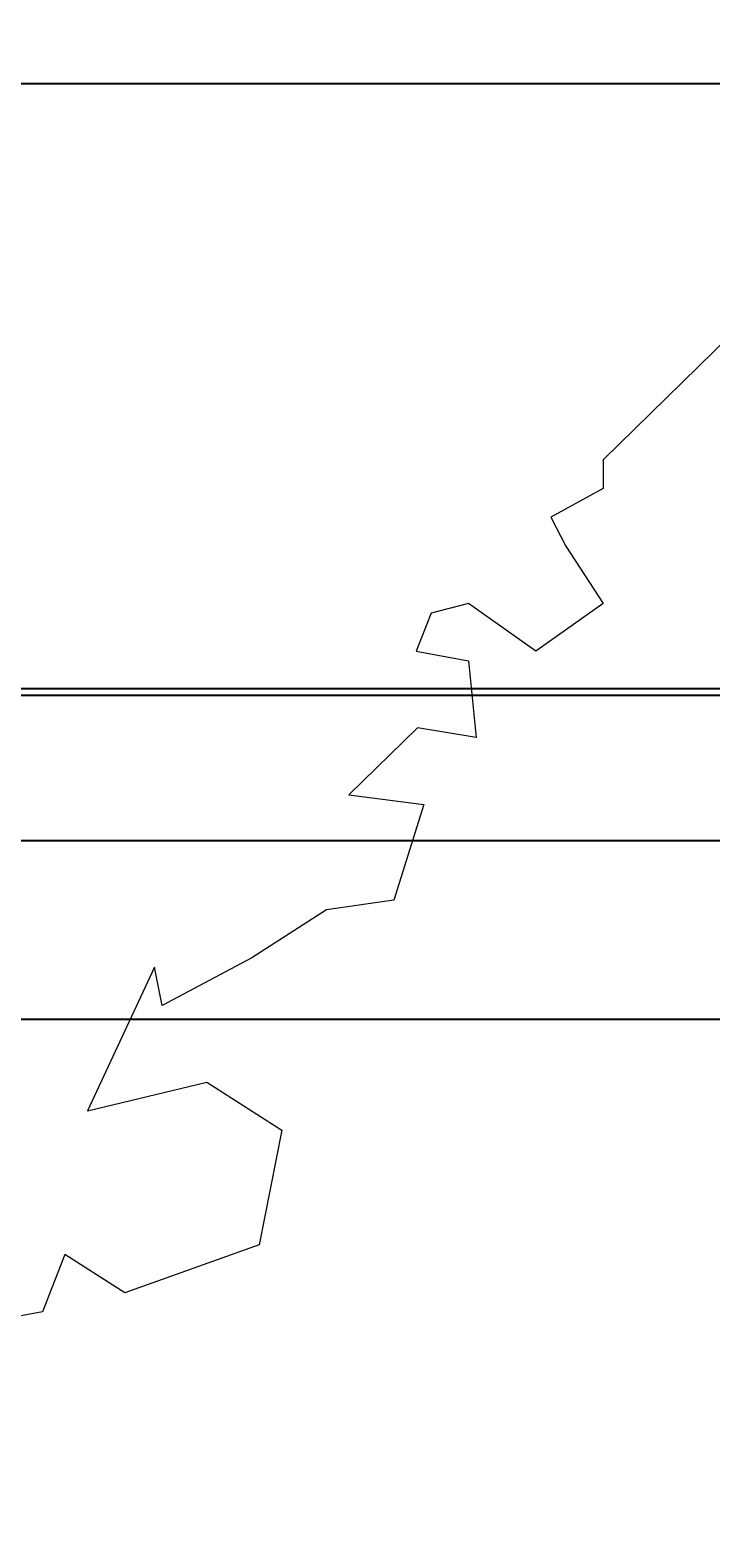
# Model space of a CAD drawing. Units: inches. Extents: x -26 to 776, y -22 to 650.
# Tile 50 of 62: x 586 to 642, y 102 to 226. Entities that reach past the tile are written whole.
import ezdxf

# ---------------------------------------------------------------- set-up
doc = ezdxf.new("R2010")
doc.units = ezdxf.units.IN
doc.header["$MEASUREMENT"] = 0
doc.layers.add('A-ANNO-DIMS', color=2, linetype='Continuous', lineweight=18)
doc.layers.add('L-PLNT-TREE', color=94, linetype='Continuous', lineweight=18)
doc.styles.get("Standard").update_dxf_attribs({"font": 'arial.ttf'})
doc.dimstyles.get("Standard").update_dxf_attribs({"dimtxt": 0.5625, "dimasz": 0.18, "dimexe": 0.18, "dimexo": 0.0625, "dimgap": 0.09, "dimtad": 0, "dimtih": 1, "dimtoh": 1, "dimdec": 4, "dimzin": 0, "dimdsep": 46, "dimlunit": 4, "dimtxsty": 'Standard', "dimcen": 0.09, "dimadec": 0, "dimazin": 0, "dimtfac": 1, "dimtdec": 4, "dimtofl": 0, "dimtmove": 0, "dimatfit": 3, "dimfxl": 1, "dimtolj": 1, "dimtzin": 0, "dimarcsym": 0})

# ---------------------------------------------------------------- blocks, each defined once
blk = doc.blocks.new('Tree - type 3 evergreen elevation')
blk.add_lwpolyline([(0.4313, 130.5029), (-6.9015, 123.3141), (-6.9015, 121.6552), (-9.9208, 119.9963), (-9.0581, 118.3373), (-6.9015, 115.0195), (-10.7835, 112.2546), (-14.6656, 115.0195), (-16.8222, 114.4665), (-17.6849, 112.2546), (-14.6656, 111.7016), (-14.2342, 107.2778), (-17.6065, 107.8307), (-21.5669, 103.9599), (-17.2536, 103.4069), (-18.9789, 97.8771), (-22.8609, 97.3241), (-27.1743, 94.5593), (-32.3504, 91.7944), (-32.7817, 94.0063), (-36.6638, 85.7116), (-29.7624, 87.3705), (-25.449, 84.6056), (-26.743, 77.9699), (-34.507, 75.205), (-37.9578, 77.4169), (-39.2518, 74.099), (-42.2711, 73.5461)])
blk = doc.blocks.new('*D20')
at = {"layer": 'A-ANNO-DIMS', "color": 0, "lineweight": -2, "transparency": 16777216}
for p, q in [((425.81, 455.47), (775.34, 455.47)), ((775.16, 455.29), (775.16, 235.85)), ((775.16, 15.66), (775.16, 235.1)), ((425.81, 15.48), (775.34, 15.48))]:
    blk.add_line(p, q, dxfattribs=at)
at = {"layer": 'A-ANNO-DIMS', "color": 0, "transparency": 16777216}
for points in [[(775.13, 455.29), (775.19, 455.29), (775.16, 455.47)], [(775.13, 15.66), (775.19, 15.66), (775.16, 15.48)]]:
    blk.add_solid(points, dxfattribs=at)
at = {"layer": 'Defpoints', "color": 0, "transparency": 16777216}
for p in [(425.74, 455.47), (775.16, 455.47), (425.74, 15.48)]:
    blk.add_point(p, dxfattribs=at)
at = {"layer": 'A-ANNO-DIMS', "color": 0, "transparency": 16777216, "insert": (775.16, 235.48), "char_height": 0.562, "attachment_point": 5}
blk.add_mtext('\\A1;440', dxfattribs=at)
blk = doc.blocks.new('*D26')
at = {"layer": 'A-ANNO-DIMS', "color": 0, "lineweight": -2, "transparency": 16777216}
for p, q in [((91.71, 171.97), (775.34, 171.97)), ((775.16, 171.79), (775.16, 166.11)), ((775.16, 159.66), (775.16, 165.35)), ((82.2, 159.48), (775.34, 159.48))]:
    blk.add_line(p, q, dxfattribs=at)
at = {"layer": 'A-ANNO-DIMS', "color": 0, "transparency": 16777216}
for points in [[(775.13, 171.79), (775.19, 171.79), (775.16, 171.97)], [(775.13, 159.66), (775.19, 159.66), (775.16, 159.48)]]:
    blk.add_solid(points, dxfattribs=at)
at = {"layer": 'Defpoints', "color": 0, "transparency": 16777216}
for p in [(91.64, 171.97), (775.16, 171.97), (82.13, 159.48)]:
    blk.add_point(p, dxfattribs=at)
at = {"layer": 'A-ANNO-DIMS', "color": 0, "transparency": 16777216, "insert": (775.16, 165.73), "char_height": 0.562, "attachment_point": 5}
blk.add_mtext('\\A1;12.49', dxfattribs=at)
blk = doc.blocks.new('*D28')
at = {"layer": 'A-ANNO-DIMS', "color": 0, "lineweight": -2, "transparency": 16777216}
for p, q in [((285.08, 314.12), (775.34, 314.12)), ((775.16, 313.94), (775.16, 243.14)), ((775.16, 171.6), (775.16, 242.4)), ((285.08, 171.42), (775.34, 171.42))]:
    blk.add_line(p, q, dxfattribs=at)
at = {"layer": 'A-ANNO-DIMS', "color": 0, "transparency": 16777216}
for points in [[(775.13, 313.94), (775.19, 313.94), (775.16, 314.12)], [(775.13, 171.6), (775.19, 171.6), (775.16, 171.42)]]:
    blk.add_solid(points, dxfattribs=at)
at = {"layer": 'Defpoints', "color": 0, "transparency": 16777216}
for p in [(285.02, 314.12), (775.16, 314.12), (285.02, 171.42)]:
    blk.add_point(p, dxfattribs=at)
at = {"layer": 'A-ANNO-DIMS', "color": 0, "transparency": 16777216, "insert": (775.16, 242.77), "char_height": 0.562, "attachment_point": 5}
blk.add_mtext('\\A1;142.7', dxfattribs=at)
blk = doc.blocks.new('*D30')
at = {"layer": 'A-ANNO-DIMS', "color": 0, "lineweight": -2, "transparency": 16777216}
for p, q in [((280.68, 144.84), (775.34, 144.84)), ((775.16, 144.66), (775.16, 86.01)), ((775.16, 26.6), (775.16, 85.25)), ((280.68, 26.42), (775.34, 26.42))]:
    blk.add_line(p, q, dxfattribs=at)
at = {"layer": 'A-ANNO-DIMS', "color": 0, "transparency": 16777216}
for points in [[(775.13, 144.66), (775.19, 144.66), (775.16, 144.84)], [(775.13, 26.6), (775.19, 26.6), (775.16, 26.42)]]:
    blk.add_solid(points, dxfattribs=at)
at = {"layer": 'Defpoints', "color": 0, "transparency": 16777216}
for p in [(280.62, 144.84), (775.16, 144.84), (280.62, 26.42)]:
    blk.add_point(p, dxfattribs=at)
at = {"layer": 'A-ANNO-DIMS', "color": 0, "transparency": 16777216, "insert": (775.16, 85.63), "char_height": 0.562, "attachment_point": 5}
blk.add_mtext('\\A1;118.41', dxfattribs=at)
blk = doc.blocks.new('*D41')
at = {"layer": 'A-ANNO-DIMS', "color": 0, "lineweight": -2, "transparency": 16777216}
for p, q in [((11.17, 221.64), (775.34, 221.64)), ((775.16, 221.46), (775.16, 190.94)), ((775.16, 159.66), (775.16, 190.18)), ((11.17, 159.48), (775.34, 159.48))]:
    blk.add_line(p, q, dxfattribs=at)
at = {"layer": 'A-ANNO-DIMS', "color": 0, "transparency": 16777216}
for points in [[(775.13, 221.46), (775.19, 221.46), (775.16, 221.64)], [(775.13, 159.66), (775.19, 159.66), (775.16, 159.48)]]:
    blk.add_solid(points, dxfattribs=at)
at = {"layer": 'Defpoints', "color": 0, "transparency": 16777216}
for p in [(11.11, 221.64), (775.16, 221.64), (11.11, 159.48)]:
    blk.add_point(p, dxfattribs=at)
at = {"layer": 'A-ANNO-DIMS', "color": 0, "transparency": 16777216, "insert": (775.16, 190.56), "char_height": 0.562, "attachment_point": 5}
blk.add_mtext('\\A1;62.16', dxfattribs=at)
blk = doc.blocks.new('*D42')
at = {"layer": 'A-ANNO-DIMS', "color": 0, "lineweight": -2, "transparency": 16777216}
for p, q in [((285.08, 171.42), (775.34, 171.42)), ((775.16, 171.24), (775.16, 165.83)), ((775.16, 159.66), (775.16, 165.07)), ((289.3, 159.48), (775.34, 159.48))]:
    blk.add_line(p, q, dxfattribs=at)
at = {"layer": 'A-ANNO-DIMS', "color": 0, "transparency": 16777216}
for points in [[(775.13, 171.24), (775.19, 171.24), (775.16, 171.42)], [(775.13, 159.66), (775.19, 159.66), (775.16, 159.48)]]:
    blk.add_solid(points, dxfattribs=at)
at = {"layer": 'Defpoints', "color": 0, "transparency": 16777216}
for p in [(285.02, 171.42), (775.16, 171.42), (289.24, 159.48)]:
    blk.add_point(p, dxfattribs=at)
at = {"layer": 'A-ANNO-DIMS', "color": 0, "transparency": 16777216, "insert": (775.16, 165.45), "char_height": 0.562, "attachment_point": 5}
blk.add_mtext('\\A1;11.935', dxfattribs=at)
blk = doc.blocks.new('*D45')
at = {"layer": 'A-ANNO-DIMS', "color": 0, "lineweight": -2, "transparency": 16777216}
for p, q in [((507.74, 408.64), (775.34, 408.64)), ((775.16, 408.46), (775.16, 212.44)), ((775.16, 15.66), (775.16, 211.68)), ((586, 15.48), (775.34, 15.48))]:
    blk.add_line(p, q, dxfattribs=at)
at = {"layer": 'A-ANNO-DIMS', "color": 0, "transparency": 16777216}
for points in [[(775.13, 408.46), (775.19, 408.46), (775.16, 408.64)], [(775.13, 15.66), (775.19, 15.66), (775.16, 15.48)]]:
    blk.add_solid(points, dxfattribs=at)
at = {"layer": 'Defpoints', "color": 0, "transparency": 16777216}
for p in [(507.68, 408.64), (775.16, 408.64), (585.94, 15.48)]:
    blk.add_point(p, dxfattribs=at)
at = {"layer": 'A-ANNO-DIMS', "color": 0, "transparency": 16777216, "insert": (775.16, 212.06), "char_height": 0.562, "attachment_point": 5}
blk.add_mtext('\\A1;393.16', dxfattribs=at)
blk = doc.blocks.new('*D48')
at = {"layer": 'A-ANNO-DIMS', "color": 0, "lineweight": -2, "transparency": 16777216}
for p, q in [((545.03, 67.41), (545.03, 649.86)), ((738.75, 50.91), (738.75, 649.86)), ((545.21, 649.68), (640.88, 649.68)), ((738.57, 649.68), (642.9, 649.68))]:
    blk.add_line(p, q, dxfattribs=at)
at = {"layer": 'A-ANNO-DIMS', "color": 0, "transparency": 16777216}
for points in [[(545.21, 649.71), (545.21, 649.65), (545.03, 649.68)], [(738.57, 649.71), (738.57, 649.65), (738.75, 649.68)]]:
    blk.add_solid(points, dxfattribs=at)
at = {"layer": 'Defpoints', "color": 0, "transparency": 16777216}
for p in [(738.75, 649.68), (545.03, 67.35), (738.75, 50.85)]:
    blk.add_point(p, dxfattribs=at)
at = {"layer": 'A-ANNO-DIMS', "color": 0, "transparency": 16777216, "insert": (641.89, 649.68), "char_height": 0.562, "attachment_point": 5}
blk.add_mtext('\\A1;193.7', dxfattribs=at)

msp = doc.modelspace()

# ---------------------------------------------------------------- block references
at = {"layer": 'L-PLNT-TREE', "xscale": 1.421226385586178, "yscale": 1.421226385586178, "zscale": 1.421226385586178}
msp.add_blockref('Tree - type 3 evergreen elevation', (642.5048, 15.4824), dxfattribs=at)

# ---------------------------------------------------------------- dimensions: what is measured, and where the dimension line sits
at = {"layer": 'A-ANNO-DIMS'}
dim = msp.add_linear_dim(base=(738.7503, 649.6763), p1=(545.0331, 67.3523), p2=(738.7503, 50.8482), dimstyle='Standard', override={"dimdec": 1, "dimlfac": 1, "dimrnd": 0, "dimzin": 0, "dimdsep": 46, "dimlunit": 2}, dxfattribs=at)
dim.commit()
dim.dimension.update_dxf_attribs({"geometry": '*D48', "text_midpoint": (641.8917, 649.6763)})
for base, p1, p2, override, picture, middle in [((775.1553, 455.4717), (425.7434, 15.4824), (425.7434, 455.4717), {"dimdec": 0, "dimlfac": 1, "dimrnd": 0, "dimzin": 0, "dimdsep": 46, "dimlunit": 2}, '*D20', (775.1553, 235.477)), ((775.1553, 408.6389), (585.9354, 15.4824), (507.6759, 408.6389), {"dimdec": 2, "dimlfac": 1, "dimrnd": 0, "dimzin": 0, "dimdsep": 46, "dimlunit": 2}, '*D45', (775.1553, 212.0606)), ((775.1553, 314.119), (285.0179, 171.4173), (285.0179, 314.119), {"dimdec": 1, "dimlfac": 1, "dimrnd": 0, "dimzin": 0, "dimdsep": 46, "dimlunit": 2}, '*D28', (775.1553, 242.7682)), ((775.1553, 221.6413), (11.1074, 159.4824), (11.1074, 221.6413), {"dimdec": 2, "dimlfac": 1, "dimrnd": 0, "dimzin": 0, "dimdsep": 46, "dimlunit": 2}, '*D41', (775.1553, 190.5618)), ((775.1553, 171.9734), (82.134, 159.4824), (91.6448, 171.9734), {"dimdec": 2, "dimlfac": 1, "dimrnd": 0, "dimzin": 0, "dimdsep": 46, "dimlunit": 2}, '*D26', (775.1553, 165.7279)), ((775.1553, 171.4173), (289.2424, 159.4824), (285.0179, 171.4173), {"dimdec": 3, "dimlfac": 1, "dimrnd": 0, "dimzin": 0, "dimdsep": 46, "dimlunit": 2}, '*D42', (775.1553, 165.4498)), ((775.1553, 144.8359), (280.6173, 26.4239), (280.6173, 144.8359), {"dimdec": 2, "dimlfac": 1, "dimrnd": 0, "dimzin": 0, "dimdsep": 46, "dimlunit": 2}, '*D30', (775.1553, 85.6299))]:
    dim = msp.add_linear_dim(base=base, p1=p1, p2=p2, angle=90, dimstyle='Standard', override=override, dxfattribs=at)
    dim.commit()
    dim.dimension.update_dxf_attribs({"geometry": picture, "text_midpoint": middle})

doc.saveas('drawing.dxf')
